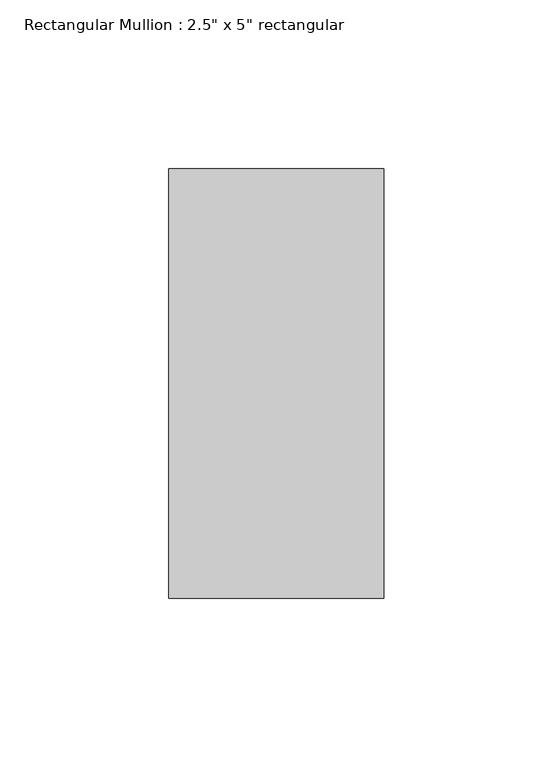
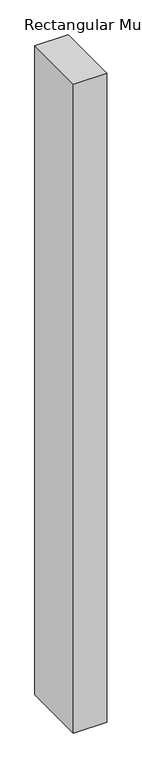
"""IFC4 building model written with IfcOpenShell, lengths in millimetres: member geometry."""

from ifc_helpers import new_model, si_unit, frame, origin, place, context, project, spatial, polyline, outline, extrude, source, transform, mapped, element, save


def member_1e564621(model_context):
    return source(origin(), model_context, "Body", "SweptSolid", [
        extrude(outline(polyline([(31.75, 63.5), (31.75, -63.5), (-31.75, -63.5), (-31.75, 63.5), (31.75, 63.5)])), frame((0.0, 0.0, -1308.0999998), z_axis=(0.0, 0.0, 1.0), x_axis=(1.0, 0.0, 0.0)), (0.0, 0.0, 1.0), 1308.0999998),
    ])


if __name__ == "__main__":
    model = new_model("IFC4")
    model_context = context("Model", 3, world=origin())
    ifc_project = project(units=[si_unit("LENGTHUNIT", "METRE", prefix="MILLI")], contexts=[model_context])
    site = spatial("IfcSite", under=ifc_project)
    building = spatial("IfcBuilding", under=site)
    placement = place(None, origin())
    member_shape = member_1e564621(model_context)
    element("IfcMember", 1, ObjectType="Rectangular Mullion : 2.5\" x 5\" rectangular", at=placement, inside=building, context=model_context, shape_type="MappedRepresentation", body=[
        mapped(member_shape, transform((0.0, 0.0, 0.0), x_axis=(1.0, 0.0, 0.0), y_axis=(0.0, 1.0, 0.0), z_axis=(0.0, 0.0, 1.0))),
    ])
    save(model, "model.ifc")

# Revit data of these elements
# Type "Rectangular Mullion : 2.5\" x 5\" rectangular"
#   built-in parameter 1007304 = 0.416667 (stored number, unit not read)
#   built-in parameter 1007301 = 0.104167 (stored number, unit not read)
#   built-in parameter 1007300 = 0.104167 (stored number, unit not read)
# Element 1 (IfcMember, "Rectangular Mullion : 2.5\" x 5\" rectangular")
#   Materials on its faces: "Aluminum"
# Materials
#   "Aluminum": class "Metal", colour RGB 247 247 247, transparency 0, Description = "Aluminum 6061", Cost = 0
